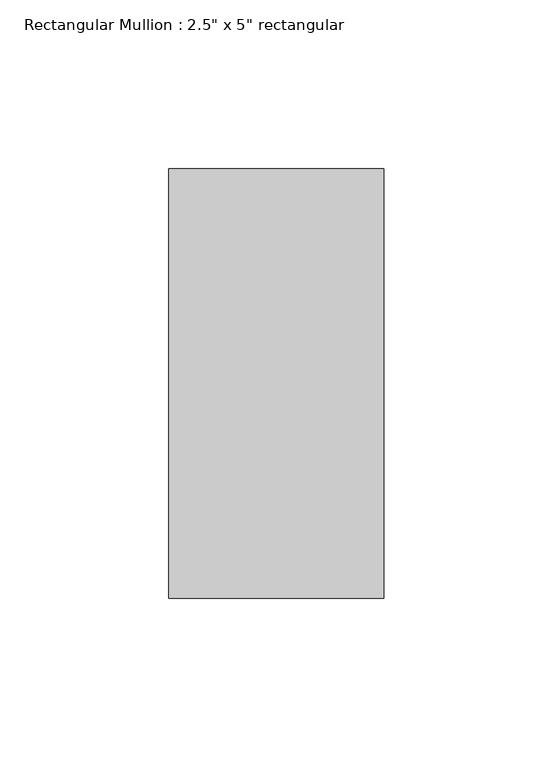
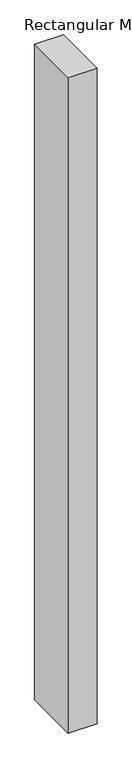
"""IFC4 building model written with IfcOpenShell, lengths in millimetres: member geometry."""

from ifc_helpers import new_model, si_unit, frame, origin, place, context, project, spatial, polyline, outline, extrude, source, transform, mapped, element, save


def member_4491d118(model_context):
    return source(origin(), model_context, "Body", "SweptSolid", [
        extrude(outline(polyline([(0.0, 63.5), (0.0, -63.5), (-63.5, -63.5), (-63.5, 63.5), (0.0, 63.5)])), frame((0.0, 0.0, -1524.0), z_axis=(0.0, 0.0, 1.0), x_axis=(1.0, 0.0, 0.0)), (0.0, 0.0, 1.0), 1524.0),
    ])


if __name__ == "__main__":
    model = new_model("IFC4")
    model_context = context("Model", 3, world=origin())
    ifc_project = project(units=[si_unit("LENGTHUNIT", "METRE", prefix="MILLI")], contexts=[model_context])
    site = spatial("IfcSite", under=ifc_project)
    building = spatial("IfcBuilding", under=site)
    placement = place(None, origin())
    member_shape = member_4491d118(model_context)
    element("IfcMember", 1, ObjectType="Rectangular Mullion : 2.5\" x 5\" rectangular", at=placement, inside=building, context=model_context, shape_type="MappedRepresentation", body=[
        mapped(member_shape, transform((0.0, 0.0, 0.0), x_axis=(1.0, 0.0, 0.0), y_axis=(0.0, 1.0, 0.0), z_axis=(0.0, 0.0, 1.0))),
    ])
    save(model, "model.ifc")

# Revit data of these elements
# Type "Rectangular Mullion : 2.5\" x 5\" rectangular"
#   built-in parameter 1007304 = 0.416667 (stored number, unit not read)
#   built-in parameter 1007301 = 0.104167 (stored number, unit not read)
#   built-in parameter 1007300 = 0.104167 (stored number, unit not read)
# Element 1 (IfcMember, "Rectangular Mullion : 2.5\" x 5\" rectangular")
#   Materials on its faces: "Rectangle 1 sq"
# Materials
#   "Rectangle 1 sq": class "Generic", colour RGB 120 120 120, transparency 0, Cost = 0
